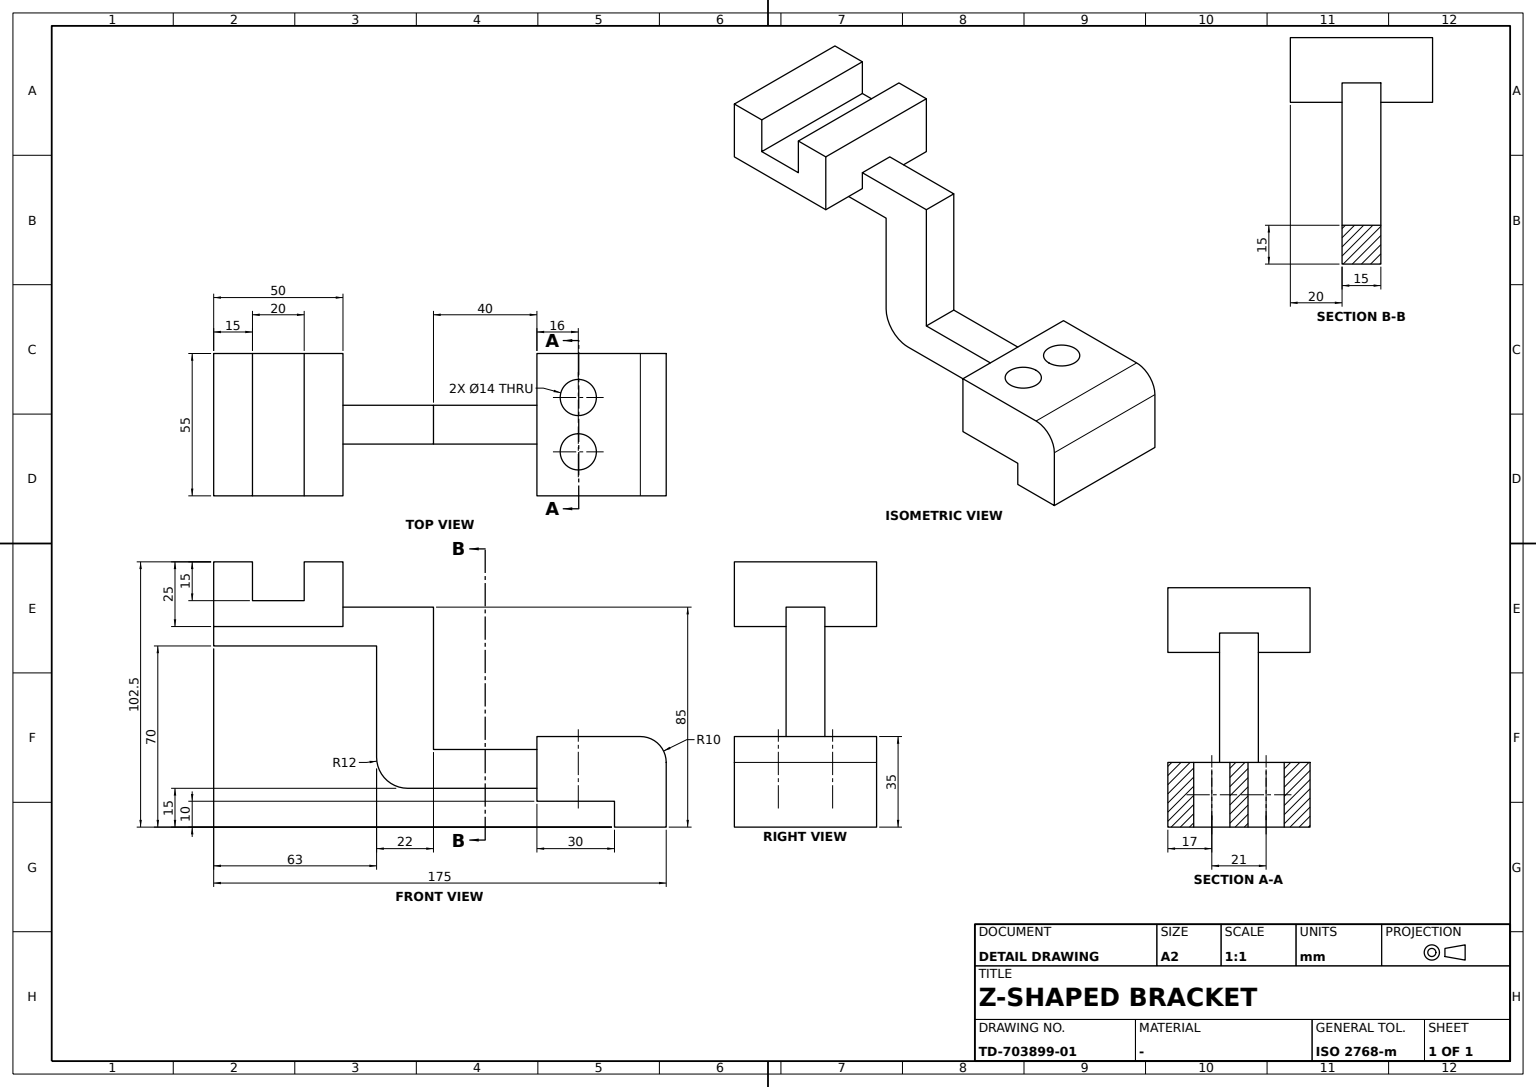
CATIA V5 part; units mm, degrees
sketch "Sketch1" plane through (0, 0, 0) normal (1, 0, 0) x (0, 1, 0)
  point P0 (62, 0)
  line L0 (62, 0) -> (0, 0)
  line L1 (0, 0) -> (0, 55)
  line L2 (0, 55) -> (-13, 55)
  point P1 (-13, 55)
  line L3 (-13, 62.5) -> (-13, 70)
  point P2 (-13, 70)
  line L4 (-13, 70) -> (22, 70)
  line L5 (22, 70) -> (22, 15)
  line L6 (22, 15) -> (62, 15)
  line L7 (62, 15) -> (62, 0)
  line L8 (-13, 55) -> (-63, 55)
  line L9 (-63, 55) -> (-63, 62.5)
  line L10 (-63, 62.5) -> (-13, 62.5)
  dimension "length L6" = 40
  dimension "distance L1 L5" = 22
  dimension "length L5" = 55
  dimension "length L7" = 15
  dimension "length L9" = 7.5
  dimension "distance P1 P2" = 15
  dimension "length L10" = 50
  dimension "distance L1 L9" = 63
  constraint coincidence P0 x-axis
  constraint horizontal L0 x-axis
  constraint horizontal L2 x-axis
  constraint horizontal L4 x-axis
  constraint horizontal L6 x-axis
  constraint horizontal L8 x-axis
  constraint horizontal L10 x-axis
  constraint vertical L1 y-axis
  constraint vertical L3 y-axis
  constraint vertical L5 y-axis
  constraint vertical L7 y-axis
  constraint vertical L9 y-axis
extrude "Pad1" add sketch "Sketch1" along normal mid plane 15
sketch "Sketch2" plane through (0, 0, 0) normal (1, 0, 0) x (0, 1, 0)
  line L0 (62, 20) -> (112, 20)
  line L1 (112, 20) -> (112, -15)
  line L2 (112, -15) -> (92, -15)
  line L3 (92, -15) -> (92, -5)
  line L4 (92, -5) -> (62, -5)
  line L5 (62, -5) -> (62, 20)
  line L6 (62, 0) -> (62, 15) construction
  line L7 (62, 15) -> (22, 15) construction
  dimension "distance L6 L5" = 0
  dimension "length L5" = 25
  dimension "length L0" = 50
  dimension "distance L7 L0" = 5
  dimension "length L4" = 30
  dimension "length L1" = 35
  constraint horizontal L0 x-axis
  constraint horizontal L2 x-axis
  constraint horizontal L4 x-axis
  constraint vertical L1 y-axis
  constraint vertical L3 y-axis
  constraint vertical L5 y-axis
extrude "Pad2" add sketch "Sketch2" along normal mid plane 55
fillet "Fillet1" radius 10 1 edges at (0, 112, 20)
fillet "Fillet2" radius 12 1 edges at (0, 0, 0)
sketch "Sketch3" plane through (0, 0, 20) normal (0, 0, 1) x (1, 0, 0)
  line L0 (-10.5, 78) -> (10.5, 78) construction
  point P0 (-10.5, 78)
  point P1 (10.5, 78)
  line L1 (-27.5, 62) -> (27.5, 62) construction
  circle A0 centre (-10.5, 78) radius 7
  circle A1 centre (10.5, 78) radius 7
  dimension "length L0" = 21
  dimension "distance L0 L1" = 16
  dimension "radius A1" = 7
  dimension "radius A0" = 7
  constraint horizontal L0 x-axis
  constraint symmetry P0 P1 y-axis
extrude "Pocket1" cut sketch "Sketch3" against normal through all
sketch "Sketch4" plane through (0, 0, 0) normal (1, 0, 0) x (0, 1, 0)
  line L0 (-13, 87.5) -> (-13, 62.5)
  line L1 (-13, 62.5) -> (-63, 62.5)
  line L2 (-63, 62.5) -> (-63, 87.5)
  line L3 (-63, 87.5) -> (-48, 87.5)
  line L4 (-48, 87.5) -> (-48, 72.5)
  line L5 (-48, 72.5) -> (-28, 72.5)
  line L6 (-28, 72.5) -> (-28, 87.5)
  point P0 (-28, 87.5)
  line L7 (-28, 87.5) -> (-13, 87.5)
  line L8 (-13, 70) -> (-13, 62.5) construction
  line L9 (-13, 62.5) -> (-63, 62.5) construction
  line L10 (-63, 62.5) -> (-63, 55) construction
  dimension "distance L0 L8" = 0
  dimension "distance L1 L9" = 0
  dimension "distance L2 L10" = 0
  dimension "length L5" = 20
  dimension "length L3" = 15
  dimension "length L4" = 15
  dimension "length L2" = 25
  constraint vertical L0 y-axis
  constraint vertical L2 y-axis
  constraint vertical L4 y-axis
  constraint vertical L6 y-axis
  constraint horizontal L1 x-axis
  constraint horizontal L3 x-axis
  constraint horizontal L5 x-axis
  constraint horizontal L7 x-axis
  constraint coincidence P0 L3
extrude "Pad3" add sketch "Sketch4" along normal mid plane 55
properties part number "14"
